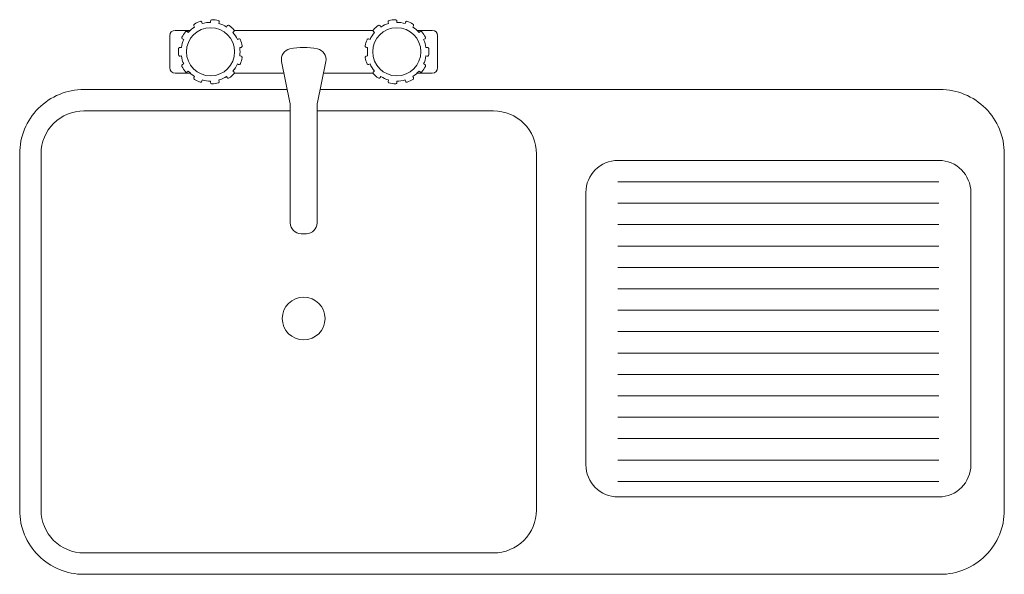
# Model space of a CAD drawing. Units: inches. Extents: x 20 to 32681, y 45 to 3082.
# Tile 5 of 5: x 31991 to 32681, y 2693 to 3082. Entities that reach past the tile are written whole.
import ezdxf

# ---------------------------------------------------------------- set-up
doc = ezdxf.new("R2010")
doc.units = ezdxf.units.IN
doc.header["$MEASUREMENT"] = 0
doc.layers.add('A-FLOR-FIXT', color=8, linetype='Continuous', lineweight=18)

# ---------------------------------------------------------------- blocks, each defined once
blk = doc.blocks.new('TARJA2')
for p, q in [((-0.09987, -0.00872), (-0.10053, -0.00769)), ((-0.09275, -0.00546), (-0.0931, -0.00429)), ((-0.08501, -0.00435), (-0.08501, -0.00313)), ((-0.07726, -0.00546), (-0.07691, -0.00429)), ((-0.07014, -0.00872), (-0.06948, -0.00769)), ((0.07408, -0.00872), (0.07341, -0.00769)), ((0.0812, -0.00546), (0.08085, -0.00429)), ((0.08894, -0.00435), (0.08894, -0.00313)), ((0.09669, -0.00546), (0.09703, -0.00429)), ((0.10381, -0.00872), (0.10447, -0.00769)), ((-0.12315, -0.01685), (-0.12315, -0.04685)), ((-0.11815, -0.01185), (-0.10388, -0.01185)), ((-0.10579, -0.01384), (-0.10671, -0.01304)), ((-0.06422, -0.01384), (-0.0633, -0.01304)), ((-0.06289, -0.01185), (0.06683, -0.01185)), ((0.06816, -0.01384), (0.06724, -0.01304)), ((0.12209, -0.01185), (0.10782, -0.01185)), ((0.10973, -0.01384), (0.11065, -0.01304)), ((0.12709, -0.01685), (0.12709, -0.04685)), ((-0.11002, -0.02043), (-0.11113, -0.01992)), ((-0.05999, -0.02043), (-0.05888, -0.01992)), ((0.06393, -0.02043), (0.06282, -0.01992)), ((0.11396, -0.02043), (0.11507, -0.01992)), ((-0.11223, -0.02794), (-0.11344, -0.02776)), ((-0.11223, -0.03576), (-0.11344, -0.03594)), ((-0.05779, -0.02794), (-0.05658, -0.02776)), ((-0.05779, -0.03576), (-0.05658, -0.03594)), ((0.06172, -0.02794), (0.06051, -0.02776)), ((0.06172, -0.03576), (0.06051, -0.03594)), ((0.11616, -0.02794), (0.11737, -0.02776)), ((0.11616, -0.03576), (0.11737, -0.03594)), ((-0.11002, -0.04327), (-0.11113, -0.04378)), ((-0.05999, -0.04327), (-0.05888, -0.04378)), ((-0.01093, -0.07925), (-0.01869, -0.04095)), ((0.01487, -0.07925), (0.02263, -0.04095)), ((0.06393, -0.04327), (0.06282, -0.04378)), ((0.11396, -0.04327), (0.11507, -0.04378)), ((-0.11815, -0.05185), (-0.10388, -0.05185)), ((-0.10579, -0.04986), (-0.10671, -0.05066)), ((-0.09987, -0.05499), (-0.10053, -0.05601)), ((-0.07014, -0.05499), (-0.06948, -0.05601)), ((-0.06422, -0.04986), (-0.0633, -0.05066)), ((-0.06289, -0.05185), (-0.01648, -0.05185)), ((0.02042, -0.05185), (0.06683, -0.05185)), ((0.06816, -0.04986), (0.06724, -0.05066)), ((0.07408, -0.05499), (0.07341, -0.05601)), ((0.10381, -0.05499), (0.10447, -0.05601)), ((0.12209, -0.05185), (0.10782, -0.05185)), ((0.10973, -0.04986), (0.11065, -0.05066)), ((-0.09275, -0.05824), (-0.0931, -0.05941)), ((-0.08501, -0.05935), (-0.08501, -0.06057)), ((-0.07726, -0.05824), (-0.07691, -0.05941)), ((0.0812, -0.05824), (0.08085, -0.05941)), ((0.08894, -0.05935), (0.08894, -0.06057)), ((0.09669, -0.05824), (0.09703, -0.05941)), ((-0.01053, -0.08322), (-0.01053, -0.19185)), ((0.01447, -0.08322), (0.01447, -0.19185)), ((0.5952, -0.13341), (0.29558, -0.13341)), ((0.5952, -0.15341), (0.29558, -0.15341)), ((0.26558, -0.16341), (0.26558, -0.41784)), ((0.6252, -0.41784), (0.6252, -0.16341)), ((0.5952, -0.17341), (0.29558, -0.17341)), ((-0.00053, -0.20185), (0.00447, -0.20185)), ((0.5952, -0.19341), (0.29558, -0.19341)), ((0.5952, -0.21341), (0.29558, -0.21341)), ((0.5952, -0.23341), (0.29558, -0.23341)), ((0.5952, -0.25341), (0.29558, -0.25341)), ((0.5952, -0.27341), (0.29558, -0.27341)), ((0.5952, -0.29341), (0.29558, -0.29341)), ((0.5952, -0.31341), (0.29558, -0.31341)), ((0.5952, -0.33341), (0.29558, -0.33341)), ((0.5952, -0.35341), (0.29558, -0.35341)), ((0.5952, -0.37341), (0.29558, -0.37341)), ((0.5952, -0.39341), (0.29558, -0.39341)), ((0.5952, -0.41341), (0.29558, -0.41341)), ((0.5952, -0.43341), (0.29558, -0.43341)), ((0.29558, -0.44784), (0.5952, -0.44784))]:
    blk.add_line(p, q)
for points in [[(0.01733, -0.06711), (0.59645, -0.06711, -0.414214), (0.65645, -0.12711), (0.65645, -0.46021, -0.414214), (0.59645, -0.52021), (-0.20332, -0.52021, -0.414214), (-0.26332, -0.46021), (-0.26332, -0.12711, -0.414214)], [(-0.26332, -0.12711, -0.414214), (-0.20332, -0.06711), (-0.01339, -0.06711, -0.414214)], [(0.01447, -0.08711), (0.17935, -0.08711, -0.414214), (0.21935, -0.12711), (0.21935, -0.46021, -0.414214), (0.17935, -0.50021), (-0.20332, -0.50021, -0.414214), (-0.24332, -0.46021), (-0.24332, -0.12711, -0.414214)], [(-0.24332, -0.12711, -0.414214), (-0.20332, -0.08711), (-0.01053, -0.08711, -0.414214)]]:
    blk.add_lwpolyline(points, format="xyb")
for centre, radius in [((-0.08501, -0.03185), 0.0225), ((0.08894, -0.03185), 0.0225), ((0.00197, -0.28117), 0.02)]:
    blk.add_circle(centre, radius)
for centre, radius, start, end in [((-0.08501, -0.03185), 0.0275, 122.72727, 139.09091), ((-0.09948, -0.00701), 0.00125, 120.23537, 212.72727), ((-0.08501, -0.03185), 0.03, 108.85554, 120.23537), ((-0.0943, -0.00464), 0.00125, 16.36364, 108.85554), ((-0.08501, -0.03185), 0.0275, 90, 106.36364), ((-0.08376, -0.00313), 0.00125, 87.50809, 180), ((-0.08501, -0.03185), 0.03, 76.12827, 87.50809), ((-0.07811, -0.00394), 0.00125, 343.63636, 76.12827), ((-0.08501, -0.03185), 0.0275, 57.27273, 73.63636), ((-0.06843, -0.00836), 0.00125, 54.78082, 147.27273), ((-0.08501, -0.03185), 0.03, 43.401, 54.78082), ((0.08894, -0.03185), 0.03, 125.21918, 136.599), ((0.07236, -0.00836), 0.00125, 32.72727, 125.21918), ((0.08894, -0.03185), 0.0275, 106.36364, 122.72727), ((0.08205, -0.00394), 0.00125, 103.87173, 196.36364), ((0.08894, -0.03185), 0.03, 92.49191, 103.87173), ((0.08769, -0.00313), 0.00125, 0, 92.49191), ((0.08894, -0.03185), 0.0275, 73.63636, 90), ((0.09823, -0.00464), 0.00125, 71.14446, 163.63636), ((0.08894, -0.03185), 0.03, 59.76463, 71.14446), ((0.08894, -0.03185), 0.0275, 40.90909, 57.27273), ((0.10342, -0.00701), 0.00125, 327.27273, 59.76463), ((-0.11815, -0.01685), 0.005, 90, 180), ((-0.11061, -0.01878), 0.00125, 152.96264, 245.45455), ((-0.08501, -0.03185), 0.03, 141.58282, 152.96264), ((-0.10753, -0.01399), 0.00125, 49.09091, 141.58282), ((-0.08501, -0.03185), 0.0275, 24.54545, 40.90909), ((-0.06412, -0.0121), 0.00125, 310.90909, 43.401), ((0.08894, -0.03185), 0.0275, 139.09091, 155.45455), ((0.06805, -0.0121), 0.00125, 136.599, 229.09091), ((0.11147, -0.01399), 0.00125, 38.41718, 130.90909), ((0.08894, -0.03185), 0.03, 27.03736, 38.41718), ((0.11455, -0.01878), 0.00125, 294.54545, 27.03736), ((0.12209, -0.01685), 0.005, 0, 90), ((-0.08501, -0.03185), 0.0275, 155.45455, 171.81818), ((-0.05836, -0.02106), 0.00125, 22.05355, 114.54545), ((-0.08501, -0.03185), 0.03, 10.67372, 22.05355), ((-0.05675, -0.02653), 0.00125, 278.18182, 10.67372), ((0.06069, -0.02653), 0.00125, 169.32628, 261.81818), ((0.08894, -0.03185), 0.03, 157.94645, 169.32628), ((0.0623, -0.02106), 0.00125, 65.45455, 157.94645), ((0.08894, -0.03185), 0.0275, 8.18182, 24.54545), ((-0.08501, -0.03185), 0.03, 174.31009, 185.68991), ((-0.11361, -0.029), 0.00125, 81.81818, 174.31009), ((-0.11361, -0.0347), 0.00125, 185.68991, 278.18182), ((-0.08501, -0.03185), 0.0275, 188.18182, 204.54545), ((-0.08501, -0.03185), 0.0275, 351.81818, 8.18182), ((-0.05675, -0.03718), 0.00125, 349.32628, 81.81818), ((-0.00889, -0.03896), 0.01, 101.1605, 191.45267), ((0.00197, -0.09399), 0.06609, 78.8395, 101.1605), ((0.01282, -0.03896), 0.01, 348.54733, 78.8395), ((0.06069, -0.03718), 0.00125, 98.18182, 190.67372), ((0.08894, -0.03185), 0.0275, 171.81818, 188.18182), ((0.08894, -0.03185), 0.0275, 335.45455, 351.81818), ((0.11755, -0.029), 0.00125, 5.68991, 98.18182), ((0.11755, -0.0347), 0.00125, 261.81818, 354.31009), ((0.08894, -0.03185), 0.03, 354.31009, 5.68991), ((-0.11061, -0.04492), 0.00125, 114.54545, 207.03736), ((-0.08501, -0.03185), 0.03, 207.03736, 218.41718), ((-0.08501, -0.03185), 0.0275, 319.09091, 335.45455), ((-0.05836, -0.04265), 0.00125, 245.45455, 337.94645), ((-0.08501, -0.03185), 0.03, 337.94645, 349.32628), ((0.08894, -0.03185), 0.03, 190.67372, 202.05355), ((0.0623, -0.04265), 0.00125, 202.05355, 294.54545), ((0.08894, -0.03185), 0.0275, 204.54545, 220.90909), ((0.08894, -0.03185), 0.03, 321.58282, 332.96264), ((0.11455, -0.04492), 0.00125, 332.96264, 65.45455), ((-0.11815, -0.04685), 0.005, 180, 270), ((-0.10753, -0.04972), 0.00125, 218.41718, 310.90909), ((-0.08501, -0.03185), 0.0275, 220.90909, 237.27273), ((-0.08501, -0.03185), 0.0275, 286.36364, 302.72727), ((-0.08501, -0.03185), 0.03, 305.21918, 316.599), ((-0.06412, -0.0516), 0.00125, 316.599, 49.09091), ((0.06805, -0.0516), 0.00125, 130.90909, 223.401), ((0.08894, -0.03185), 0.03, 223.401, 234.78082), ((0.08894, -0.03185), 0.0275, 237.27273, 253.63636), ((0.08894, -0.03185), 0.0275, 302.72727, 319.09091), ((0.11147, -0.04972), 0.00125, 229.09091, 321.58282), ((0.12209, -0.04685), 0.005, 270, 360), ((-0.09948, -0.05669), 0.00125, 147.27273, 239.76463), ((-0.08501, -0.03185), 0.03, 239.76463, 251.14446), ((-0.0943, -0.05906), 0.00125, 251.14446, 343.63636), ((-0.08501, -0.03185), 0.0275, 253.63636, 270), ((-0.08376, -0.06057), 0.00125, 180, 272.49191), ((-0.08501, -0.03185), 0.03, 272.49191, 283.87173), ((-0.07811, -0.05976), 0.00125, 283.87173, 16.36364), ((-0.06843, -0.05534), 0.00125, 212.72727, 305.21918), ((0.07236, -0.05534), 0.00125, 234.78082, 327.27273), ((0.08205, -0.05976), 0.00125, 163.63636, 256.12827), ((0.08894, -0.03185), 0.03, 256.12827, 267.50809), ((0.08769, -0.06057), 0.00125, 267.50809, 360), ((0.08894, -0.03185), 0.0275, 270, 286.36364), ((0.09823, -0.05906), 0.00125, 196.36364, 288.85554), ((0.08894, -0.03185), 0.03, 288.85554, 300.23537), ((0.10342, -0.05669), 0.00125, 300.23537, 32.72727), ((-0.03053, -0.08322), 0.02, 0, 11.45267), ((-0.02053, -0.08221), 0.01, 0, 11.45267), ((0.03447, -0.08322), 0.02, 168.54733, 180), ((0.29558, -0.16341), 0.03, 90, 180), ((0.5952, -0.16341), 0.03, 0, 90), ((-0.00053, -0.19185), 0.01, 180, 270), ((0.00447, -0.19185), 0.01, 270, 360), ((0.29558, -0.41784), 0.03, 180, 270), ((0.5952, -0.41784), 0.03, 270, 360)]:
    blk.add_arc(centre, radius, start, end)

msp = doc.modelspace()

# ---------------------------------------------------------------- block references
at = {"layer": 'A-FLOR-FIXT', "xscale": 750, "yscale": 750, "zscale": 750}
msp.add_blockref('TARJA2', (32188.19, 3083.04), dxfattribs=at)

doc.saveas('drawing.dxf')
